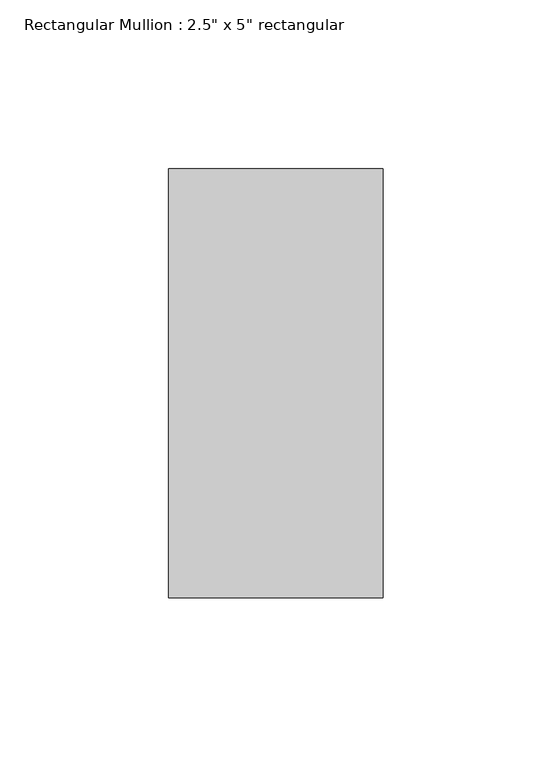
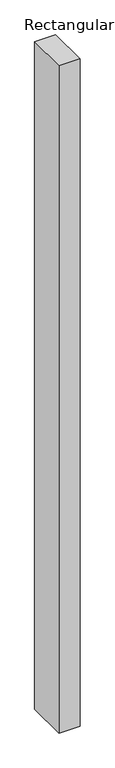
"""IFC4 building model written with IfcOpenShell, lengths in millimetres: member geometry."""

from ifc_helpers import new_model, si_unit, frame, origin, place, context, project, spatial, polyline, outline, extrude, source, transform, mapped, element, save


def member_7cbddb58(model_context):
    return source(origin(), model_context, "Body", "SweptSolid", [
        extrude(outline(polyline([(31.75, 63.5), (31.75, -63.5), (-31.75, -63.5), (-31.75, 63.5), (31.75, 63.5)])), frame((0.0, 0.0, -2133.6), z_axis=(0.0, 0.0, 1.0), x_axis=(1.0, 0.0, 0.0)), (0.0, 0.0, 1.0), 2133.6),
    ])


if __name__ == "__main__":
    model = new_model("IFC4")
    model_context = context("Model", 3, world=origin())
    ifc_project = project(units=[si_unit("LENGTHUNIT", "METRE", prefix="MILLI")], contexts=[model_context])
    site = spatial("IfcSite", under=ifc_project)
    building = spatial("IfcBuilding", under=site)
    placement = place(None, origin())
    member_shape = member_7cbddb58(model_context)
    element("IfcMember", 1, ObjectType="Rectangular Mullion : 2.5\" x 5\" rectangular", at=placement, inside=building, context=model_context, shape_type="MappedRepresentation", body=[
        mapped(member_shape, transform((0.0, 0.0, 0.0), x_axis=(1.0, 0.0, 0.0), y_axis=(0.0, 1.0, 0.0), z_axis=(0.0, 0.0, 1.0))),
    ])
    save(model, "model.ifc")

# Revit data of these elements
# Type "Rectangular Mullion : 2.5\" x 5\" rectangular"
#   built-in parameter 1007304 = 0.416667 (stored number, unit not read)
#   built-in parameter 1007301 = 0.104167 (stored number, unit not read)
#   built-in parameter 1007300 = 0.104167 (stored number, unit not read)
# Element 1 (IfcMember, "Rectangular Mullion : 2.5\" x 5\" rectangular")
#   Materials on its faces: "Aluminum"
# Materials
#   "Aluminum": class "Metal", colour RGB 247 247 247, transparency 0, Description = "Aluminum 6061", Cost = 0
